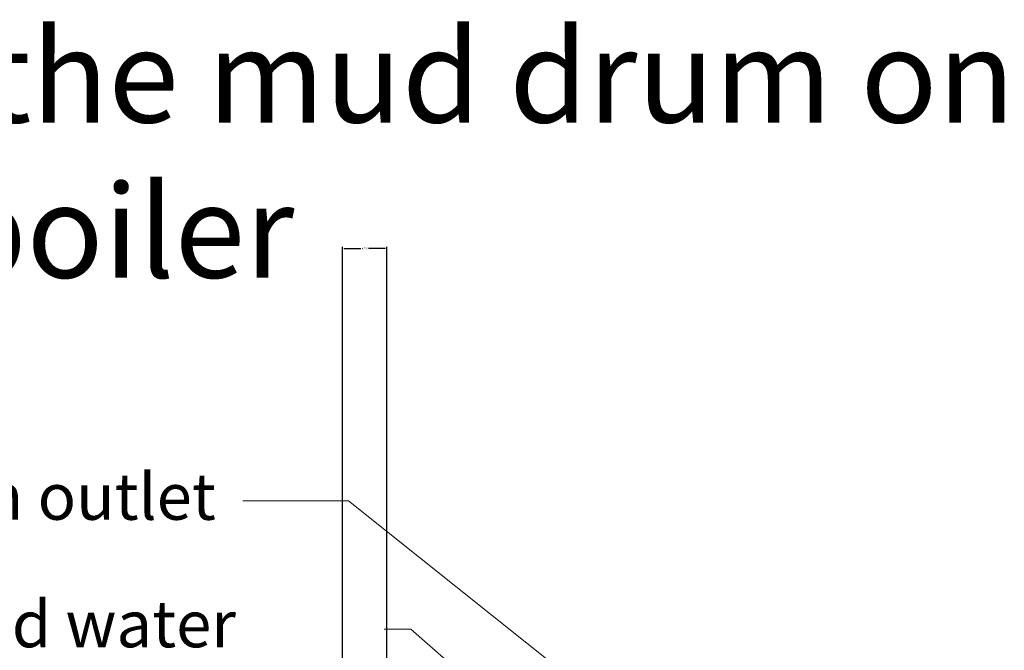
# Model space of a CAD drawing. Units: inches. Extents: x -1 to 292, y -3 to 199.
# Tile 52 of 52: x 181 to 286, y 131 to 199. Entities that reach past the tile are written whole.
import ezdxf

# ---------------------------------------------------------------- set-up
doc = ezdxf.new("R2010")
doc.units = ezdxf.units.IN
doc.header["$MEASUREMENT"] = 0
for name, color, linetype, lineweight in [('M-ANNO-LEAD', 2, 'Continuous', 18), ('M-ANNO-TEXT', 3, 'Continuous', 25), ('M-DIMS', 2, 'Continuous', 18)]:
    doc.layers.add(name, color=color, linetype=linetype, lineweight=lineweight)
doc.styles.get("Standard").update_dxf_attribs({"font": 'arial.ttf'})
doc.dimstyles.get("Standard").update_dxf_attribs({"dimtxt": 0.18, "dimasz": 0.18, "dimexe": 0.18, "dimexo": 0.0625, "dimgap": 0.09, "dimtad": 0, "dimtih": 1, "dimtoh": 1, "dimdec": 4, "dimzin": 0, "dimdsep": 46, "dimtxsty": 'Standard', "dimcen": 0.09, "dimadec": 0, "dimazin": 0, "dimtfac": 1, "dimtdec": 4, "dimtofl": 0, "dimtmove": 0, "dimatfit": 3, "dimfxl": 1, "dimtolj": 1, "dimtzin": 0, "dimarcsym": 0})

# ---------------------------------------------------------------- blocks, each defined once
blk = doc.blocks.new('*D27')
at = {"layer": 'Defpoints', "color": 0, "transparency": 16777216}
for p in [(220.03, 174.36), (215.24, 88.13), (220.03, 85.36)]:
    blk.add_point(p, dxfattribs=at)
at = {"layer": 'M-DIMS', "color": 0, "lineweight": -2, "transparency": 16777216}
for p, q in [((215.24, 88.19), (215.24, 174.54)), ((220.03, 85.43), (220.03, 174.54)), ((215.42, 174.36), (217.24, 174.36)), ((219.85, 174.36), (218.03, 174.36))]:
    blk.add_line(p, q, dxfattribs=at)
at = {"layer": 'M-DIMS', "color": 0, "transparency": 16777216}
for points in [[(215.42, 174.39), (215.42, 174.33), (215.24, 174.36)], [(219.85, 174.39), (219.85, 174.33), (220.03, 174.36)]]:
    blk.add_solid(points, dxfattribs=at)
at = {"layer": 'M-DIMS', "color": 0, "transparency": 16777216, "insert": (217.64, 174.36), "char_height": 0.18, "attachment_point": 5}
blk.add_mtext('\\A1;4.793', dxfattribs=at)

msp = doc.modelspace()

# ---------------------------------------------------------------- linework, layer by layer
at = {"layer": 'M-ANNO-LEAD'}
for p, q in [((215.8975, 147.2795), (204.5604, 147.2795)), ((242.9552, 125.7269), (215.8975, 147.2795)), ((222.6022, 133.5105), (219.7228, 133.5105)), ((234.9209, 122.7118), (222.6022, 133.5105))]:
    msp.add_line(p, q, dxfattribs=at)

# ---------------------------------------------------------------- texts
at = {"layer": 'M-ANNO-TEXT', "attachment_point": 1}
for s, width, heights, insert, char_height in [('\\pxqc;diagram of the location of the mud drum on a  water tube boiler', 286.43424, [43.6883], (5.3019, 197.8921), 10), ('steam outlet', 40.442607, [0], (161.2863, 150.2478), 5), ('feed water inlet', 47.899539, [0], (169.9729, 136.5612), 5)]:
    msp.add_mtext_dynamic_manual_height_columns(s, width=width, gutter_width=1, heights=heights, dxfattribs=dict(at, insert=insert, char_height=char_height))

# ---------------------------------------------------------------- dimensions: what is measured, and where the dimension line sits
at = {"layer": 'M-DIMS'}
dim = msp.add_linear_dim(base=(220.034, 174.3627), p1=(215.2407, 88.1304), p2=(220.034, 85.363), dimstyle='Standard', override={"dimdec": 3, "dimlfac": 1, "dimrnd": 0, "dimzin": 0, "dimdsep": 46, "dimlunit": 2}, dxfattribs=at)
dim.commit()
dim.dimension.update_dxf_attribs({"geometry": '*D27', "text_midpoint": (217.6374, 174.3627)})

doc.saveas('drawing.dxf')
